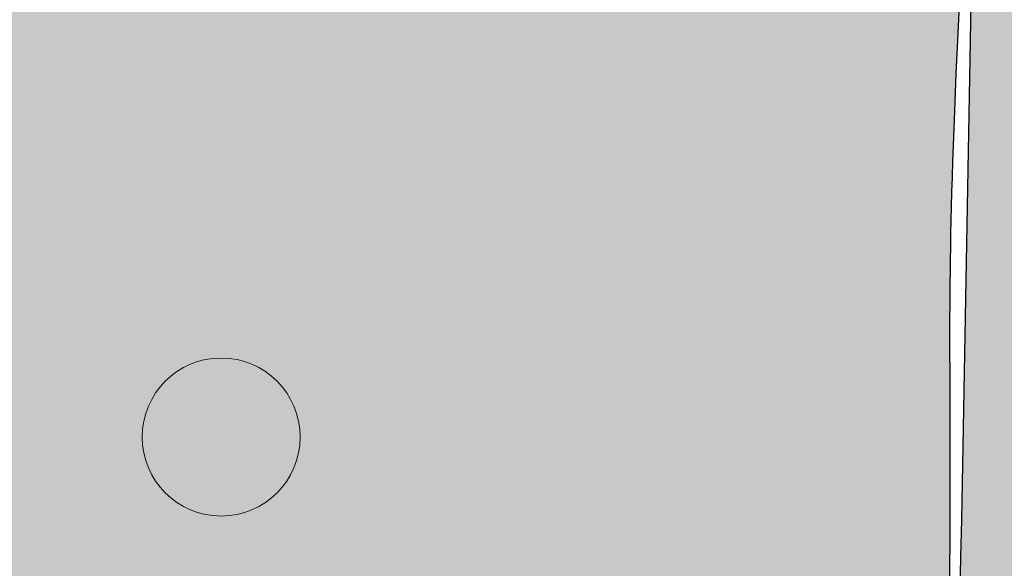
# Model space of a CAD drawing. Units: millimetres. Extents: x 11032 to 26788, y 3406 to 24505.
# Tile 58 of 78: x 16358 to 17293, y 15498 to 16019. Entities that reach past the tile are written whole.
import ezdxf

# ---------------------------------------------------------------- set-up
doc = ezdxf.new("R2010")
doc.units = ezdxf.units.MM
doc.header["$MEASUREMENT"] = 0
for name, color, linetype, lineweight in [('A-ANNO-DIMS', 2, 'Continuous', 18), ('A-ELEV-GUIT', 7, 'Continuous', 18), ('A-ROOF', 7, 'Continuous', 30), ('A-WALL', 7, 'Continuous', 35), ('E-LITE', 7, 'Continuous', 18), ('E-LITE-PATT', 7, 'Continuous', 13)]:
    doc.layers.add(name, color=color, linetype=linetype, lineweight=lineweight)
doc.layers.add('A-ROOF-PATT', color=9, linetype='Continuous', lineweight=13, true_color=0xc7c8ca)
doc.styles.get("Standard").update_dxf_attribs({"font": 'arial.ttf'})
doc.dimstyles.get("Standard").update_dxf_attribs({"dimtxt": 150, "dimasz": 100, "dimexe": 10, "dimexo": 5, "dimgap": 5, "dimtad": 0, "dimtih": 1, "dimtoh": 1, "dimdec": 0, "dimzin": 0, "dimdsep": 46, "dimtxsty": 'Standard', "dimcen": 0.09, "dimadec": 0, "dimazin": 0, "dimtfac": 1, "dimtdec": 0, "dimtofl": 0, "dimtmove": 0, "dimatfit": 3, "dimfxl": 1, "dimtolj": 1, "dimtzin": 0, "dimarcsym": 0})

# ---------------------------------------------------------------- blocks, each defined once
blk = doc.blocks.new('RECESSED-LIGHT-150')
blk.add_circle((75, 75), 75)
blk = doc.blocks.new('*D36')
at = {"layer": 'A-ANNO-DIMS', "color": 0, "lineweight": -2, "transparency": 16777216}
for p, q in [((12301.26, 17115.89), (12301.26, 24416.86)), ((25397.4, 4466.4), (25397.4, 24416.86)), ((12401.26, 24406.86), (18569.2, 24406.86)), ((25297.4, 24406.86), (19129.47, 24406.86))]:
    blk.add_line(p, q, dxfattribs=at)
at = {"layer": 'A-ANNO-DIMS', "color": 0, "transparency": 16777216}
for points in [[(12401.26, 24423.52), (12401.26, 24390.19), (12301.26, 24406.86)], [(25297.4, 24423.52), (25297.4, 24390.19), (25397.4, 24406.86)]]:
    blk.add_solid(points, dxfattribs=at)
at = {"layer": 'Defpoints', "color": 0, "transparency": 16777216}
for p in [(25397.4, 24406.86), (12301.26, 17110.89), (25397.4, 4461.4)]:
    blk.add_point(p, dxfattribs=at)
at = {"layer": 'A-ANNO-DIMS', "color": 0, "transparency": 16777216, "insert": (18849.33, 24406.86), "char_height": 150, "attachment_point": 5}
blk.add_mtext('\\A1;13096', dxfattribs=at)
blk = doc.blocks.new('*D37')
at = {"layer": 'A-ANNO-DIMS', "color": 0, "lineweight": -2, "transparency": 16777216}
for p, q in [((18087.74, 23450.36), (11334.76, 23450.36)), ((11344.76, 23350.36), (11344.76, 14037.46)), ((11344.76, 4561.4), (11344.76, 13874.29)), ((12927.66, 4461.4), (11334.76, 4461.4))]:
    blk.add_line(p, q, dxfattribs=at)
at = {"layer": 'A-ANNO-DIMS', "color": 0, "transparency": 16777216}
for points in [[(11328.1, 23350.36), (11361.43, 23350.36), (11344.76, 23450.36)], [(11328.1, 4561.4), (11361.43, 4561.4), (11344.76, 4461.4)]]:
    blk.add_solid(points, dxfattribs=at)
at = {"layer": 'Defpoints', "color": 0, "transparency": 16777216}
for p in [(11344.76, 23450.36), (18092.74, 23450.36), (12932.66, 4461.4)]:
    blk.add_point(p, dxfattribs=at)
at = {"layer": 'A-ANNO-DIMS', "color": 0, "transparency": 16777216, "insert": (11344.76, 13955.88), "char_height": 150, "attachment_point": 5}
blk.add_mtext('\\A1;18989', dxfattribs=at)
blk = doc.blocks.new('*D57')
at = {"layer": 'A-ANNO-DIMS', "color": 0, "lineweight": -2, "transparency": 16777216}
for p, q in [((14994.7, 7266.4), (14994.7, 24416.86)), ((20894.7, 7266.4), (20894.7, 24416.86)), ((15094.7, 24406.86), (17715.98, 24406.86)), ((20794.7, 24406.86), (18173.42, 24406.86))]:
    blk.add_line(p, q, dxfattribs=at)
at = {"layer": 'A-ANNO-DIMS', "color": 0, "transparency": 16777216}
for points in [[(15094.7, 24423.52), (15094.7, 24390.19), (14994.7, 24406.86)], [(20794.7, 24423.52), (20794.7, 24390.19), (20894.7, 24406.86)]]:
    blk.add_solid(points, dxfattribs=at)
at = {"layer": 'Defpoints', "color": 0, "transparency": 16777216}
for p in [(20894.7, 24406.86), (14994.7, 7261.4), (20894.7, 7261.4)]:
    blk.add_point(p, dxfattribs=at)
at = {"layer": 'A-ANNO-DIMS', "color": 0, "transparency": 16777216, "insert": (17944.7, 24406.86), "char_height": 150, "attachment_point": 5}
blk.add_mtext('\\A1;5900', dxfattribs=at)

msp = doc.modelspace()

# ---------------------------------------------------------------- hatches: boundary and pattern name
at = {"layer": 'A-ROOF-PATT'}
h = msp.add_hatch(color=256, dxfattribs=at)
edge = h.paths.add_edge_path()
edge.add_spline(control_points=[(17532.827, 17324.837), (17391.335, 17349.016), (16840.872, 17494.912), (16080.055, 18069.544), (14738.803, 18299.641), (13382.429, 18838.336), (12580.532, 17870.207), (12430.422, 17563.822)], knot_values=[2977.6027945, 2977.6027945, 2977.6027945, 2977.6027945, 3438.1840601, 4811.6463022, 5622.8675483, 7588.0288188, 8560.6685791, 8560.6685791, 8560.6685791, 8560.6685791], degree=3, periodic=0)
edge.add_spline(control_points=[(12430.422, 17563.822), (12437.904, 17573.36), (12445.386, 17582.899), (12452.869, 17592.437), (12452.869, 17592.438), (12452.869, 17592.438), (12452.869, 17592.438)], knot_values=[1408.564138, 1408.564138, 1408.564138, 1408.564138, 1444.85989, 1444.85989, 1444.85989, 1444.8601183, 1444.8601183, 1444.8601183, 1444.8601183], degree=3, periodic=0)
edge.add_spline(control_points=[(12452.869, 17592.438), (12555.432, 17723.185), (12736.557, 17929.686), (13044.86, 18114.643), (13219.943, 18189.644), (13299.92, 18220.646)], knot_values=[339.318246, 339.318246, 339.318246, 339.318246, 836.8349967, 1151.2512933, 1408.564138, 1408.564138, 1408.564138, 1408.564138], degree=3, periodic=0)
edge.add_spline(control_points=[(13299.92, 18220.646), (13299.998, 18220.689), (13300.077, 18220.732), (13319.738, 18231.488), (13339.24, 18241.402), (13388.645, 18264.703), (13418.466, 18277.069), (13478.019, 18298.648), (13507.751, 18307.861), (13544.561, 18317.488), (13551.584, 18319.245), (13558.612, 18320.924)], knot_values=[3783.8950972, 3783.8950972, 3783.8950972, 3783.8950972, 3784.1737101, 3784.1737101, 3853.4666747, 3853.4666747, 3960.2401917, 3960.2401917, 4067.0137087, 4067.0137087, 4092.1744649, 4092.1744649, 4092.1744649, 4092.1744649], degree=3, periodic=0)
edge.add_spline(control_points=[(13558.612, 18320.924), (13581.407, 18326.373), (13604.25, 18331.007), (13657.184, 18339.957), (13687.338, 18343.732), (13748.098, 18348.892), (13778.704, 18350.276), (13840.46, 18350.833), (13871.609, 18350.005), (13934.496, 18346.313), (13966.232, 18343.449), (14030.297, 18335.871), (14062.625, 18331.158), (14127.853, 18320.088), (14160.753, 18313.73), (14241.357, 18296.556), (14289.343, 18284.997), (14386.31, 18259.688), (14435.291, 18245.941), (14534.161, 18217.034), (14584.049, 18201.875), (14684.682, 18170.964), (14735.427, 18155.212), (14837.763, 18123.971), (14889.354, 18108.482), (14954.971, 18089.677), (14968.586, 18085.823), (14992.391, 18079.184), (15002.566, 18076.376), (15021.739, 18071.153), (15030.731, 18068.729), (15047.707, 18064.21), (15055.694, 18062.106), (15079.815, 18055.825), (15095.905, 18051.728), (15143.966, 18039.717), (15175.729, 18032.084), (15254.84, 18013.501), (15301.798, 18002.866), (15394.186, 17981.845), (15439.615, 17971.459), (15528.833, 17950.135), (15572.62, 17939.197), (15658.477, 17916.021), (15700.546, 17903.785), (15753.633, 17886.734), (15765.446, 17882.835), (15786.574, 17875.653), (15795.915, 17872.404), (15810.108, 17867.349), (15814.99, 17865.588), (15824.736, 17862.029), (15829.611, 17860.226), (15844.241, 17854.75), (15854.002, 17851.008), (15883.312, 17839.521), (15902.885, 17831.512), (15966.355, 17804.548), (16010.39, 17784.302), (16098.838, 17741.267), (16143.25, 17718.478), (16232.497, 17671.098), (16277.332, 17646.507), (16367.515, 17596.295), (16412.862, 17570.676), (16504.202, 17519.209), (16550.194, 17493.362), (16643.009, 17442.263), (16689.831, 17417.011), (16756.517, 17382.472), (16775.937, 17372.58), (16795.455, 17362.84)], knot_values=[4092.1744649, 4092.1744649, 4092.1744649, 4092.1744649, 4173.7872258, 4173.7872258, 4280.5607428, 4280.5607428, 4387.3342598, 4387.3342598, 4494.1077768, 4494.1077768, 4600.8812939, 4600.8812939, 4707.6548109, 4707.6548109, 4814.4283279, 4814.4283279, 4967.1262405, 4967.1262405, 5119.8241531, 5119.8241531, 5272.5220657, 5272.5220657, 5425.2199783, 5425.2199783, 5577.9178908, 5577.9178908, 5617.7853319, 5617.7853319, 5647.4648479, 5647.4648479, 5673.611025, 5673.611025, 5696.747607, 5696.747607, 5743.6818903, 5743.6818903, 5837.5504571, 5837.5504571, 5979.7261046, 5979.7261046, 6121.9017521, 6121.9017521, 6264.0773996, 6264.0773996, 6406.2530471, 6406.2530471, 6447.2585849, 6447.2585849, 6480.0420882, 6480.0420882, 6497.3077062, 6497.3077062, 6514.5733242, 6514.5733242, 6549.1045602, 6549.1045602, 6618.1670322, 6618.1670322, 6772.6610171, 6772.6610171, 6927.155002, 6927.155002, 7081.6489869, 7081.6489869, 7236.1429718, 7236.1429718, 7390.6369567, 7390.6369567, 7545.1309416, 7545.1309416, 7608.1992868, 7608.1992868, 7608.1992868, 7608.1992868], degree=3, periodic=0)
edge.add_spline(control_points=[(16795.455, 17362.84), (16814.335, 17349.456), (16832.897, 17336.263), (16873.225, 17307.197), (16894.778, 17291.386), (16936.221, 17259.941), (16956.11, 17244.308), (16993.863, 17213.094), (17011.726, 17197.514), (17041.993, 17169.265), (17054.791, 17156.601), (17078.762, 17131.225), (17089.933, 17118.516), (17110.618, 17092.991), (17120.131, 17080.178), (17130.17, 17065.264), (17131.487, 17063.277), (17133.77, 17059.776), (17134.746, 17058.261), (17136.69, 17055.205), (17137.657, 17053.668), (17140.539, 17049.025), (17142.438, 17045.89), (17148.068, 17036.367), (17151.732, 17029.859), (17163.03, 17008.788), (17170.335, 16993.646), (17184.087, 16961.978), (17190.534, 16945.453), (17202.562, 16911.165), (17208.142, 16893.402), (17218.448, 16856.821), (17223.173, 16838.003), (17231.801, 16799.51), (17235.705, 16779.837), (17241.533, 16746.739), (17243.676, 16733.5), (17247.718, 16706.37), (17249.608, 16692.472), (17252.066, 16672.69), (17252.761, 16666.875), (17254.1, 16655.226), (17254.744, 16649.4), (17256.596, 16631.917), (17257.727, 16620.254), (17260.823, 16585.238), (17262.489, 16561.858), (17266.551, 16488.654), (17267.658, 16438.661), (17267.349, 16375.228), (17267.193, 16362.07), (17266.95, 16348.891)], knot_values=[15.1130472, 15.1130472, 15.1130472, 15.1130472, 82.6995146, 82.6995146, 165.3990291, 165.3990291, 248.0985437, 248.0985437, 330.7980583, 330.7980583, 397.9419458, 397.9419458, 465.0858333, 465.0858333, 532.2297209, 532.2297209, 542.533741, 542.533741, 550.3568158, 550.3568158, 558.1798906, 558.1798906, 573.8260402, 573.8260402, 605.1183395, 605.1183395, 672.7640614, 672.7640614, 740.4097834, 740.4097834, 808.0555054, 808.0555054, 875.7012273, 875.7012273, 943.3469493, 943.3469493, 987.6613492, 987.6613492, 1033.4121612, 1033.4121612, 1052.3850876, 1052.3850876, 1071.358014, 1071.358014, 1109.3038668, 1109.3038668, 1185.1955724, 1185.1955724, 1346.4419026, 1346.4419026, 1388.5586631, 1388.5586631, 1388.5586631, 1388.5586631], degree=3, periodic=0)
edge.add_spline(control_points=[(17266.95, 16348.891), (17266.95, 16348.891), (17266.95, 16348.891), (17266.95, 16348.891), (17253.182, 15602.417), (17239.414, 14855.943), (17225.646, 14109.469)], knot_values=[1388.5586631, 1388.5586631, 1388.5586631, 1388.5586631, 1388.5589654, 1388.5589654, 1388.5589654, 3774.0767661, 3774.0767661, 3774.0767661, 3774.0767661], degree=3, periodic=0)
edge.add_spline(control_points=[(17225.646, 14109.469), (17226.198, 14109.827), (17226.748, 14110.185), (17242.065, 14120.191), (17255.956, 14130.116), (17274.422, 14144.286), (17279.609, 14148.386), (17284.686, 14152.511)], knot_values=[1926.3423968, 1926.3423968, 1926.3423968, 1926.3423968, 1927.316729, 1927.316729, 1953.5121761, 1953.5121761, 1964.0732348, 1964.0732348, 1964.0732348, 1964.0732348], degree=3, periodic=0)
edge.add_spline(control_points=[(17284.686, 14152.511), (17315.791, 14194.761), (17384.413, 14446.273), (17407.128, 14793.401), (17407.093, 15295.84), (17423.274, 15626.362), (17415.601, 15782.507)], knot_values=[0, 0, 0, 0, 163.2554674, 619.2296767, 1171.8624483, 1621.6355562, 1621.6355562, 1621.6355562, 1621.6355562], degree=3, periodic=0)
edge.add_spline(control_points=[(17415.601, 15782.507), (17438.21, 16077.57), (17410.495, 16533.484), (17390.893, 17030.649), (17301.082, 17169.349)], knot_values=[543.9784753, 543.9784753, 543.9784753, 543.9784753, 1452.9852767, 1960.0114926, 1960.0114926, 1960.0114926, 1960.0114926], degree=3, periodic=0)
edge.add_spline(control_points=[(17301.082, 17169.349), (17346.58, 17157.64), (17392.235, 17147.336), (17467.161, 17132.609), (17496.336, 17127.412), (17525.58, 17122.709)], knot_values=[8131.593939, 8131.593939, 8131.593939, 8131.593939, 8269.7349273, 8269.7349273, 8357.5016646, 8357.5016646, 8357.5016646, 8357.5016646], degree=3, periodic=0)
edge.add_line((17525.58, 17122.709), (17532.827, 17324.837))
edge = h.paths.add_edge_path(flags=17)
edge.add_spline(control_points=[(13340.537, 14602.706), (13316.172, 14726.456), (13323.666, 14932.342), (13637.836, 15081.117), (13863.248, 15171.051), (14002.1, 15224.503), (14058.539, 15244.876)], knot_values=[680.8931862, 680.8931862, 680.8931862, 680.8931862, 1033.4728289, 1337.4008326, 1604.7214264, 1784.2944722, 1784.2944722, 1784.2944722, 1784.2944722], degree=3, periodic=0)
edge.add_spline(control_points=[(14058.539, 15244.876), (14058.289, 15275.236), (14057.634, 15305.434), (14055.312, 15376.527), (14053.359, 15417.248), (14048.642, 15497.048), (14045.89, 15536.143), (14042.888, 15574.619)], knot_values=[6573.1065419, 6573.1065419, 6573.1065419, 6573.1065419, 6636.7330012, 6636.7330012, 6723.8890547, 6723.8890547, 6809.6328771, 6809.6328771, 6809.6328771, 6809.6328771], degree=3, periodic=0)
edge.add_spline(control_points=[(14042.888, 15574.619), (13546.54, 15403.221), (13074.735, 15143.241), (13277.36, 14695.339), (13340.537, 14602.706)], knot_values=[503.7925783, 503.7925783, 503.7925783, 503.7925783, 1728.1787606, 2051.34844, 2051.34844, 2051.34844, 2051.34844], degree=3, periodic=0)
h = msp.add_hatch(color=256, dxfattribs=at)
h.set_gradient(color1=(254, 234, 185), color2=(254, 204, 102), name='HEMISPHERICAL')
edge = h.paths.add_edge_path()
edge.add_line((15084.393, 17001.32), (15284.393, 17051.32))
edge.add_line((15284.393, 17051.32), (15470.537, 16752.334))
edge.add_spline(control_points=[(15470.537, 16752.334), (15683.311, 16831.508), (16106.827, 16912.335), (16625.609, 16876.997), (17083.498, 16357.78), (17257.801, 16180.113)], knot_values=[0, 0, 0, 0, 655.2936334, 1252.0157838, 1989.6162859, 1989.6162859, 1989.6162859, 1989.6162859], degree=3, periodic=0)
edge.add_spline(control_points=[(17257.801, 16180.113), (17260.851, 16236.372), (17263.9, 16292.632), (17266.95, 16348.891)], knot_values=[1132.9967717, 1132.9967717, 1132.9967717, 1132.9967717, 1198.0464225, 1198.0464225, 1198.0464225, 1198.0464225], degree=3, periodic=0)
edge.add_spline(control_points=[(17266.95, 16348.891), (17267.193, 16362.07), (17267.349, 16375.228), (17267.658, 16438.661), (17266.551, 16488.654), (17262.489, 16561.858), (17260.823, 16585.238), (17257.727, 16620.254), (17256.596, 16631.917), (17254.744, 16649.4), (17254.1, 16655.226), (17252.761, 16666.875), (17252.066, 16672.69), (17249.608, 16692.472), (17247.718, 16706.37), (17243.676, 16733.5), (17241.533, 16746.739), (17235.705, 16779.837), (17231.801, 16799.51), (17223.173, 16838.003), (17218.448, 16856.821), (17208.142, 16893.402), (17202.562, 16911.165), (17190.534, 16945.453), (17184.087, 16961.978), (17170.335, 16993.646), (17163.03, 17008.788), (17151.732, 17029.859), (17148.068, 17036.367), (17142.438, 17045.89), (17140.539, 17049.025), (17137.657, 17053.668), (17136.69, 17055.205), (17134.746, 17058.261), (17133.77, 17059.776), (17131.487, 17063.277), (17130.17, 17065.264), (17120.131, 17080.178), (17110.618, 17092.991), (17089.933, 17118.516), (17078.762, 17131.225), (17054.791, 17156.601), (17041.993, 17169.265), (17011.726, 17197.514), (16993.863, 17213.094), (16956.11, 17244.308), (16936.221, 17259.941), (16894.778, 17291.386), (16873.225, 17307.197), (16832.897, 17336.263), (16814.335, 17349.456), (16795.455, 17362.84)], knot_values=[15.1130472, 15.1130472, 15.1130472, 15.1130472, 57.2298077, 57.2298077, 218.4761379, 218.4761379, 294.3678435, 294.3678435, 332.3136963, 332.3136963, 351.2866227, 351.2866227, 370.2595491, 370.2595491, 416.0103612, 416.0103612, 460.324761, 460.324761, 527.970483, 527.970483, 595.616205, 595.616205, 663.2619269, 663.2619269, 730.9076489, 730.9076489, 798.5533709, 798.5533709, 829.8456701, 829.8456701, 845.4918197, 845.4918197, 853.3148945, 853.3148945, 861.1379693, 861.1379693, 871.4419895, 871.4419895, 938.585877, 938.585877, 1005.7297645, 1005.7297645, 1072.8736521, 1072.8736521, 1155.5731666, 1155.5731666, 1238.2726812, 1238.2726812, 1320.9721958, 1320.9721958, 1388.5586631, 1388.5586631, 1388.5586631, 1388.5586631], degree=3, periodic=0)
edge.add_spline(control_points=[(16795.455, 17362.84), (16775.937, 17372.58), (16756.517, 17382.472), (16689.831, 17417.011), (16643.009, 17442.263), (16550.194, 17493.362), (16504.202, 17519.209), (16412.862, 17570.676), (16367.515, 17596.295), (16277.332, 17646.507), (16232.497, 17671.098), (16143.25, 17718.478), (16098.838, 17741.267), (16010.39, 17784.302), (15966.355, 17804.548), (15902.885, 17831.512), (15883.312, 17839.521), (15854.002, 17851.008), (15844.241, 17854.75), (15829.611, 17860.226), (15824.736, 17862.029), (15814.99, 17865.588), (15810.108, 17867.349), (15795.915, 17872.404), (15786.574, 17875.653), (15765.446, 17882.835), (15753.633, 17886.734), (15700.546, 17903.785), (15658.477, 17916.021), (15572.62, 17939.197), (15528.833, 17950.135), (15439.615, 17971.459), (15394.186, 17981.845), (15301.798, 18002.866), (15254.84, 18013.501), (15175.729, 18032.084), (15143.966, 18039.717), (15095.905, 18051.728), (15079.815, 18055.825), (15055.694, 18062.106), (15047.707, 18064.21), (15030.731, 18068.729), (15021.739, 18071.153), (15002.566, 18076.376), (14992.391, 18079.184), (14968.586, 18085.823), (14954.971, 18089.677), (14889.354, 18108.482), (14837.763, 18123.971), (14735.427, 18155.212), (14684.682, 18170.964), (14584.049, 18201.875), (14534.161, 18217.034), (14435.291, 18245.941), (14386.31, 18259.688), (14289.343, 18284.997), (14241.357, 18296.556), (14160.753, 18313.73), (14127.853, 18320.088), (14062.625, 18331.158), (14030.297, 18335.871), (13966.232, 18343.449), (13934.496, 18346.313), (13871.609, 18350.005), (13840.46, 18350.833), (13778.704, 18350.276), (13748.098, 18348.892), (13687.338, 18343.732), (13657.184, 18339.957), (13604.25, 18331.007), (13581.407, 18326.373), (13558.612, 18320.924)], knot_values=[4092.1744649, 4092.1744649, 4092.1744649, 4092.1744649, 4155.2428101, 4155.2428101, 4309.736795, 4309.736795, 4464.2307799, 4464.2307799, 4618.7247648, 4618.7247648, 4773.2187497, 4773.2187497, 4927.7127346, 4927.7127346, 5082.2067195, 5082.2067195, 5151.2691915, 5151.2691915, 5185.8004275, 5185.8004275, 5203.0660455, 5203.0660455, 5220.3316635, 5220.3316635, 5253.1151668, 5253.1151668, 5294.1207046, 5294.1207046, 5436.2963521, 5436.2963521, 5578.4719996, 5578.4719996, 5720.6476471, 5720.6476471, 5862.8232946, 5862.8232946, 5956.6918614, 5956.6918614, 6003.6261447, 6003.6261447, 6026.7627267, 6026.7627267, 6052.9089038, 6052.9089038, 6082.5884198, 6082.5884198, 6122.4558609, 6122.4558609, 6275.1537734, 6275.1537734, 6427.851686, 6427.851686, 6580.5495986, 6580.5495986, 6733.2475112, 6733.2475112, 6885.9454238, 6885.9454238, 6992.7189408, 6992.7189408, 7099.4924578, 7099.4924578, 7206.2659749, 7206.2659749, 7313.0394919, 7313.0394919, 7419.8130089, 7419.8130089, 7526.5865259, 7526.5865259, 7608.1992868, 7608.1992868, 7608.1992868, 7608.1992868], degree=3, periodic=0)
edge.add_spline(control_points=[(13558.612, 18320.924), (13472.381, 18287.498), (13386.15, 18254.072), (13299.92, 18220.646), (13299.92, 18220.646), (13299.92, 18220.646), (13299.92, 18220.646)], knot_values=[61.8832457, 61.8832457, 61.8832457, 61.8832457, 339.3179746, 339.3179746, 339.3179746, 339.318246, 339.318246, 339.318246, 339.318246], degree=3, periodic=0)
edge.add_spline(control_points=[(13299.92, 18220.646), (13219.943, 18189.644), (13044.86, 18114.643), (12736.557, 17929.686), (12555.432, 17723.185), (12452.869, 17592.438)], knot_values=[339.318246, 339.318246, 339.318246, 339.318246, 596.6310906, 911.0473872, 1408.564138, 1408.564138, 1408.564138, 1408.564138], degree=3, periodic=0)
edge.add_spline(control_points=[(12452.869, 17592.438), (12452.869, 17592.438), (12452.869, 17592.438), (12452.869, 17592.437), (12445.386, 17582.899), (12437.904, 17573.36), (12430.422, 17563.822)], knot_values=[1408.564138, 1408.564138, 1408.564138, 1408.564138, 1408.5643663, 1408.5643663, 1408.5643663, 1444.8601183, 1444.8601183, 1444.8601183, 1444.8601183], degree=3, periodic=0)
edge.add_spline(control_points=[(12430.422, 17563.822), (12373.797, 17448.248), (12157.302, 16836.764), (12751.985, 16393.69), (13424.325, 15907.903), (14042.888, 15574.619)], knot_values=[0, 0, 0, 0, 366.8993034, 1975.5941082, 2977.6027945, 2977.6027945, 2977.6027945, 2977.6027945], degree=3, periodic=0)
edge.add_spline(control_points=[(14042.888, 15574.619), (14042.839, 15575.252), (14042.789, 15575.886), (14039.681, 15615.607), (14036.366, 15654.052), (14029.551, 15729.305), (14026.05, 15766.114), (14019.175, 15837.686), (14015.8, 15872.45), (13903.823, 16338.596)], knot_values=[6310.2261504, 6310.2261504, 6310.2261504, 6310.2261504, 6311.6383814, 6311.6383814, 6398.7944349, 6398.7944349, 6485.9504884, 6485.9504884, 6573.1065419, 6573.1065419, 6573.1065419, 6573.1065419], degree=3, periodic=0)
edge.add_spline(control_points=[(13903.823, 16338.596), (14237.315, 16236.889), (14456.623, 16167.555), (14614.196, 16115.84)], knot_values=[0, 0, 0, 0, 202.9853419, 202.9853419, 202.9853419, 202.9853419], degree=3, periodic=0)
edge.add_spline(control_points=[(14614.196, 16115.84), (14663.209, 16178.992), (14799.965, 16341.237), (14969.915, 16481.426), (15084.393, 16556.825)], knot_values=[2405.0345045, 2405.0345045, 2405.0345045, 2405.0345045, 2644.8826966, 3039.2707272, 3039.2707272, 3039.2707272, 3039.2707272], degree=3, periodic=0)
edge.add_line((15084.393, 16556.825), (15084.393, 17001.32))
h.paths.add_polyline_path([(14195.599, 17606.181, -1), (14395.599, 17606.181, -1)], flags=16)
h.paths.add_polyline_path([(13310.178, 17032.97, -1), (13510.178, 17032.97, -1)], flags=16)
h = msp.add_hatch(color=256, dxfattribs=at)
h.set_gradient(color1=(254, 234, 185), color2=(254, 204, 102), name='HEMISPHERICAL')
edge = h.paths.add_edge_path()
edge.add_spline(control_points=[(16560.042, 14907.752), (16569.192, 14907.664), (16578.343, 14907.575), (16587.493, 14907.486), (16832.101, 14905.115), (17122.895, 14902.296), (16849.359, 14976.117), (16870.954, 15304.114), (17098.337, 15241.178), (17235.385, 15203.245)], knot_values=[0, 0, 0, 0, 14.8674385, 14.8674385, 14.8674385, 412.2943091, 487.3345915, 708.6416004, 1044.3939449, 1044.3939449, 1044.3939449, 1044.3939449], degree=3, periodic=0)
edge.add_line((16587.504, 14907.486), (16560.207, 14907.486))
edge.add_line((16560.207, 14907.486), (15784.393, 16153.61))
edge.add_line((15784.393, 16153.61), (15784.393, 15385.996))
edge.add_spline(control_points=[(15784.393, 15385.996), (15798.391, 15360.52), (15847.198, 15266.214), (15887.196, 15168.614), (15912.903, 15096.727)], knot_values=[1463.2850479, 1463.2850479, 1463.2850479, 1463.2850479, 1550.659771, 1779.9599361, 1779.9599361, 1779.9599361, 1779.9599361], degree=3, periodic=0)
edge.add_spline(control_points=[(15912.903, 15096.727), (15913.652, 15095.649), (15914.403, 15094.565), (15925.191, 15078.948), (15935.516, 15063.47), (15956.582, 15030.918), (15967.324, 15013.844), (15989.119, 14978.386), (16000.173, 14960.003), (16022.525, 14922.193), (16033.824, 14902.767), (16056.63, 14863.116), (16068.138, 14842.891), (16091.349, 14801.871), (16103.053, 14781.075), (16126.666, 14739.118), (16138.575, 14717.958), (16162.628, 14675.459), (16174.772, 14654.12), (16199.352, 14611.428), (16211.787, 14590.075), (16237.037, 14547.491), (16249.851, 14526.26), (16271.946, 14490.566), (16281.092, 14476.044), (16299.694, 14447.129), (16309.149, 14432.737), (16328.456, 14404.098), (16338.307, 14389.85), (16358.518, 14361.503), (16368.879, 14347.403), (16390.266, 14319.347), (16401.291, 14305.391), (16420.626, 14281.969), (16428.703, 14272.467), (16445.363, 14253.527), (16453.946, 14244.088), (16471.727, 14225.278), (16480.926, 14215.907), (16500.075, 14197.247), (16510.026, 14187.959), (16530.844, 14169.504), (16541.71, 14160.337), (16564.549, 14142.195), (16576.522, 14133.22), (16597.69, 14118.448), (16606.528, 14112.565), (16624.87, 14101.004), (16634.376, 14095.326), (16654.117, 14084.255), (16664.352, 14078.862), (16685.603, 14068.46), (16696.619, 14063.452), (16719.46, 14053.944), (16731.285, 14049.444), (16755.742, 14041.097), (16768.374, 14037.251), (16794.396, 14030.368), (16807.787, 14027.332), (16835.229, 14022.23), (16849.279, 14020.163), (16877.882, 14017.141), (16892.435, 14016.186), (16921.835, 14015.489), (16936.683, 14015.749), (16961.564, 14017.241), (16971.582, 14018.127), (16986.57, 14019.883), (16991.56, 14020.54), (16999.027, 14021.63), (17001.514, 14022.011), (17006.48, 14022.809), (17008.962, 14023.225), (17014.824, 14024.251), (17018.193, 14024.875), (17036.262, 14028.398), (17050.55, 14031.826), (17078.171, 14039.583), (17091.505, 14043.912), (17115.643, 14052.705), (17126.557, 14057.089), (17137.108, 14061.688)], knot_values=[2010.7639617, 2010.7639617, 2010.7639617, 2010.7639617, 2014.7029827, 2014.7029827, 2067.238337, 2067.238337, 2119.7736913, 2119.7736913, 2172.3090457, 2172.3090457, 2224.8444, 2224.8444, 2277.3797543, 2277.3797543, 2329.9151086, 2329.9151086, 2382.450463, 2382.450463, 2434.9858173, 2434.9858173, 2487.5211716, 2487.5211716, 2540.0565259, 2540.0565259, 2576.3179289, 2576.3179289, 2612.5793318, 2612.5793318, 2648.8407347, 2648.8407347, 2685.1021376, 2685.1021376, 2721.3635405, 2721.3635405, 2746.252015, 2746.252015, 2771.1404895, 2771.1404895, 2796.028964, 2796.028964, 2820.9174385, 2820.9174385, 2845.8059131, 2845.8059131, 2870.6943876, 2870.6943876, 2887.5132757, 2887.5132757, 2904.3321639, 2904.3321639, 2921.1510521, 2921.1510521, 2937.9699402, 2937.9699402, 2954.7888284, 2954.7888284, 2971.6077166, 2971.6077166, 2988.4266047, 2988.4266047, 3005.2454929, 3005.2454929, 3022.0643811, 3022.0643811, 3038.8832692, 3038.8832692, 3050.1975453, 3050.1975453, 3055.8546833, 3055.8546833, 3058.6832524, 3058.6832524, 3061.5118214, 3061.5118214, 3065.3934173, 3065.3934173, 3082.4668716, 3082.4668716, 3099.5403259, 3099.5403259, 3114.5433443, 3114.5433443, 3114.5433443, 3114.5433443], degree=3, periodic=0)
edge.add_spline(control_points=[(17137.108, 14061.688), (17165.253, 14274.398), (17209.97, 14653.885), (17230.2, 15035.586), (17235.385, 15203.245)], knot_values=[1968.0804557, 1968.0804557, 1968.0804557, 1968.0804557, 2611.5282875, 3114.5379264, 3114.5379264, 3114.5379264, 3114.5379264], degree=3, periodic=0)
edge = h.paths.add_edge_path()
edge.add_spline(control_points=[(16856.103, 14956.992), (16852.841, 14961.219), (16849.83, 14965.576), (16842.539, 14977.287), (16838.658, 14984.798), (16832.033, 15000.109), (16829.289, 15007.911), (16824.126, 15026.008), (16822.047, 15036.354), (16819.308, 15057.097), (16818.649, 15067.496), (16818.576, 15088.188), (16819.162, 15098.483), (16821.467, 15118.823), (16823.186, 15128.868), (16827.696, 15148.567), (16830.486, 15158.22), (16836.065, 15173.969), (16838.565, 15180.211), (16844.079, 15192.402), (16847.092, 15198.353), (16852.029, 15207.021), (16853.744, 15209.868), (16857.321, 15215.468), (16859.188, 15218.226), (16863.017, 15223.558), (16864.978, 15226.136), (16872.565, 15235.558), (16878.593, 15241.952), (16891.428, 15253.591), (16898.232, 15258.834), (16912.397, 15268.127), (16919.756, 15272.176), (16934.816, 15279.138), (16942.515, 15282.052), (16958.1, 15286.873), (16965.985, 15288.78), (16984.013, 15292.142), (16994.186, 15293.334), (17014.631, 15294.619), (17024.904, 15294.713), (17048.453, 15293.935), (17061.76, 15292.783), (17088.519, 15289.422), (17101.972, 15287.211), (17131.961, 15281.46), (17148.526, 15277.734), (17181.692, 15269.627), (17198.292, 15265.245), (17222.182, 15258.759), (17229.535, 15256.737), (17236.862, 15254.714)], knot_values=[9.6639535, 9.6639535, 9.6639535, 9.6639535, 20.0351668, 20.0351668, 36.9411752, 36.9411752, 53.8471837, 53.8471837, 75.7795687, 75.7795687, 97.7119538, 97.7119538, 119.6443388, 119.6443388, 141.5767238, 141.5767238, 163.5091089, 163.5091089, 178.3829945, 178.3829945, 193.2568801, 193.2568801, 200.6938229, 200.6938229, 208.1307657, 208.1307657, 215.4448585, 215.4448585, 235.5795923, 235.5795923, 255.7143261, 255.7143261, 275.8490598, 275.8490598, 295.9837936, 295.9837936, 316.1185274, 316.1185274, 341.7220543, 341.7220543, 367.3255812, 367.3255812, 400.1572431, 400.1572431, 432.988905, 432.988905, 473.0440165, 473.0440165, 513.099128, 513.099128, 530.9692999, 530.9692999, 530.9692999, 530.9692999], degree=3, periodic=0)
edge.add_spline(control_points=[(17236.862, 15254.714), (17240.377, 15387.456), (17242.496, 15609.536), (17239.752, 15831.567), (17250.544, 16044.717)], knot_values=[1250.9818616, 1250.9818616, 1250.9818616, 1250.9818616, 1649.1516581, 1916.613987, 1916.613987, 1916.613987, 1916.613987], degree=3, periodic=0)
edge.add_spline(control_points=[(17250.544, 16044.717), (17229.169, 16066.505), (17207.794, 16088.292), (17186.419, 16110.08), (17186.418, 16110.08), (17186.418, 16110.081), (17186.418, 16110.081)], knot_values=[-88.5185581, -88.5185581, -88.5185581, -88.5185581, -0.0012784, -0.0012784, -0.0012784, 0, 0, 0, 0], degree=3, periodic=0)
edge.add_spline(control_points=[(17186.418, 16110.081), (17169.261, 16127.569), (17151.499, 16145.947), (17114.892, 16184.084), (17096.046, 16203.842), (17057.437, 16244.305), (17037.673, 16265.01), (16997.415, 16306.918), (16976.921, 16328.12), (16927.79, 16378.347), (16898.924, 16407.388), (16840.771, 16464.327), (16811.484, 16492.225), (16758.449, 16540.764), (16734.666, 16561.798), (16687.634, 16601.588), (16664.382, 16620.344), (16624.116, 16650.909), (16606.897, 16663.324), (16583.769, 16678.999), (16577.49, 16683.149), (16567.144, 16689.805), (16563.039, 16692.397), (16550.823, 16699.959), (16542.775, 16704.739), (16526.841, 16713.814), (16518.956, 16718.108), (16495.524, 16730.301), (16480.199, 16737.514), (16449.97, 16750.334), (16435.066, 16755.942), (16405.476, 16765.764), (16390.79, 16769.979), (16361.418, 16777.195), (16346.731, 16780.197), (16317.147, 16785.133), (16302.249, 16787.067), (16272.053, 16789.992), (16256.756, 16790.981), (16225.609, 16792.125), (16209.759, 16792.279), (16177.385, 16791.865), (16160.862, 16791.296), (16136.98, 16790.07), (16129.942, 16789.661), (16118.22, 16788.91), (16113.574, 16788.594), (16103.645, 16787.886), (16098.362, 16787.489), (16087.761, 16786.652), (16082.439, 16786.212), (16066.413, 16784.825), (16055.649, 16783.812), (16023.135, 16780.505), (16001.164, 16777.942), (15934.539, 16769.141), (15889.17, 16761.791), (15797.417, 16743.949), (15751.033, 16733.457), (15645.217, 16705.796), (15585.74, 16687.58), (15526.207, 16666.217), (15525.367, 16665.915), (15524.528, 16665.613)], knot_values=[0, 0, 0, 0, 71.0501454, 71.0501454, 142.1002909, 142.1002909, 213.1504363, 213.1504363, 284.2005818, 284.2005818, 381.323193, 381.323193, 478.4458043, 478.4458043, 557.8219847, 557.8219847, 637.1981651, 637.1981651, 698.3122593, 698.3122593, 721.3971375, 721.3971375, 736.7790891, 736.7790891, 767.5429924, 767.5429924, 798.3068957, 798.3068957, 859.8347022, 859.8347022, 921.3625088, 921.3625088, 982.8903154, 982.8903154, 1044.4181219, 1044.4181219, 1105.9459285, 1105.9459285, 1167.4737351, 1167.4737351, 1229.0015416, 1229.0015416, 1290.5293482, 1290.5293482, 1315.8990035, 1315.8990035, 1332.3812792, 1332.3812792, 1350.9052657, 1350.9052657, 1369.4292522, 1369.4292522, 1406.4772252, 1406.4772252, 1480.5731712, 1480.5731712, 1628.7650633, 1628.7650633, 1776.9569554, 1776.9569554, 1966.3109251, 1966.3109251, 1969.019495, 1969.019495, 1969.019495, 1969.019495], degree=3, periodic=0)
edge.add_line((15524.528, 16665.613), (16587.978, 14957.484))
edge.add_spline(control_points=[(16587.978, 14957.484), (16605.253, 14957.316), (16622.516, 14957.149), (16665.945, 14956.759), (16691.933, 14956.554), (16742.419, 14956.302), (16766.918, 14956.255), (16813.531, 14956.412), (16835.647, 14956.617), (16856.103, 14956.992)], knot_values=[872.2181925, 872.2181925, 872.2181925, 872.2181925, 900.2857301, 900.2857301, 943.3659889, 943.3659889, 986.4462476, 986.4462476, 1029.5265064, 1029.5265064, 1029.5265064, 1029.5265064], degree=3, periodic=0)
h.paths.add_polyline_path([(16474.605, 15622.642, -1), (16624.605, 15622.642, -1)], flags=16)
h.paths.add_polyline_path([(16198.536, 16037.613, -1), (16348.536, 16037.613, -1)], flags=16)
h.paths.add_polyline_path([(16475.717, 16408.125, -1), (16625.717, 16408.125, -1)], flags=16)
at = {"layer": 'E-LITE-PATT'}
h = msp.add_hatch(color=256, dxfattribs=at)
h.paths.add_polyline_path([(13510.178, 17032.97, 1), (13310.178, 17032.97, 1)])
h.paths.add_polyline_path([(14395.599, 17606.181, 1), (14195.599, 17606.181, 1)])
h.paths.add_polyline_path([(16625.717, 16408.125, 1), (16475.717, 16408.125, 1)])
h.paths.add_polyline_path([(16348.536, 16037.613, 1), (16198.536, 16037.613, 1)])
h.paths.add_polyline_path([(16624.605, 15622.642, 1), (16474.605, 15622.642, 1)])
edge = h.paths.add_edge_path()
edge.add_spline(control_points=[(17236.862, 15254.714), (17229.535, 15256.737), (17222.182, 15258.759), (17198.292, 15265.245), (17181.692, 15269.627), (17148.526, 15277.734), (17131.961, 15281.46), (17101.972, 15287.211), (17088.519, 15289.422), (17061.76, 15292.783), (17048.453, 15293.935), (17024.904, 15294.713), (17014.631, 15294.619), (16994.186, 15293.334), (16984.013, 15292.142), (16965.985, 15288.78), (16958.1, 15286.873), (16942.515, 15282.052), (16934.816, 15279.138), (16919.756, 15272.176), (16912.397, 15268.127), (16898.232, 15258.834), (16891.428, 15253.591), (16878.593, 15241.952), (16872.565, 15235.558), (16864.978, 15226.136), (16863.017, 15223.558), (16859.188, 15218.226), (16857.321, 15215.468), (16853.744, 15209.868), (16852.029, 15207.021), (16847.092, 15198.353), (16844.079, 15192.402), (16838.565, 15180.211), (16836.065, 15173.969), (16830.486, 15158.22), (16827.696, 15148.567), (16823.186, 15128.868), (16821.467, 15118.823), (16819.162, 15098.483), (16818.576, 15088.188), (16818.649, 15067.496), (16819.308, 15057.097), (16822.047, 15036.354), (16824.126, 15026.008), (16829.289, 15007.911), (16832.033, 15000.109), (16838.658, 14984.798), (16842.539, 14977.287), (16849.83, 14965.576), (16852.841, 14961.219), (16856.103, 14956.992)], knot_values=[9.6639535, 9.6639535, 9.6639535, 9.6639535, 27.5341253, 27.5341253, 67.5892368, 67.5892368, 107.6443483, 107.6443483, 140.4760102, 140.4760102, 173.3076721, 173.3076721, 198.911199, 198.911199, 224.5147259, 224.5147259, 244.6494597, 244.6494597, 264.7841935, 264.7841935, 284.9189272, 284.9189272, 305.053661, 305.053661, 325.1883948, 325.1883948, 332.5024876, 332.5024876, 339.9394304, 339.9394304, 347.3763732, 347.3763732, 362.2502588, 362.2502588, 377.1241444, 377.1241444, 399.0565295, 399.0565295, 420.9889145, 420.9889145, 442.9212995, 442.9212995, 464.8536846, 464.8536846, 486.7860696, 486.7860696, 503.6920781, 503.6920781, 520.5980866, 520.5980866, 530.9692999, 530.9692999, 530.9692999, 530.9692999], degree=3, periodic=0)
edge.add_spline(control_points=[(16856.103, 14956.992), (16835.647, 14956.617), (16813.531, 14956.412), (16766.918, 14956.255), (16742.419, 14956.302), (16691.933, 14956.554), (16665.945, 14956.759), (16622.516, 14957.149), (16605.253, 14957.316), (16587.978, 14957.484)], knot_values=[872.2181925, 872.2181925, 872.2181925, 872.2181925, 915.2984513, 915.2984513, 958.37871, 958.37871, 1001.4589687, 1001.4589687, 1029.5265064, 1029.5265064, 1029.5265064, 1029.5265064], degree=3, periodic=0)
edge.add_line((16587.978, 14957.484), (16619.296, 14907.181))
edge.add_spline(control_points=[(16619.296, 14907.181), (16852.686, 14904.98), (17116.098, 14904.13), (16849.359, 14976.117), (16870.954, 15304.114), (17098.337, 15241.178), (17235.385, 15203.245)], knot_values=[0, 0, 0, 0, 380.1882376, 455.2285201, 676.535529, 1012.2878735, 1012.2878735, 1012.2878735, 1012.2878735], degree=3, periodic=0)
edge.add_spline(control_points=[(17235.385, 15203.245), (17235.916, 15220.399), (17236.408, 15237.556), (17236.862, 15254.714)], knot_values=[1916.613987, 1916.613987, 1916.613987, 1916.613987, 1968.0804557, 1968.0804557, 1968.0804557, 1968.0804557], degree=3, periodic=0)
h = msp.add_hatch(color=256, dxfattribs=at)
h.paths.add_polyline_path([(13510.178, 17032.97, 1), (13310.178, 17032.97, 1)])
h.paths.add_polyline_path([(14195.599, 17606.181, 1), (14395.599, 17606.181, 1)])
h.paths.add_polyline_path([(16625.717, 16408.125, 1), (16475.717, 16408.125, 1)])
h.paths.add_polyline_path([(16198.536, 16037.613, 1), (16348.536, 16037.613, 1)])
h.paths.add_polyline_path([(16474.605, 15622.642, 1), (16624.605, 15622.642, 1)])

# ---------------------------------------------------------------- linework, layer by layer
at = {"layer": 'A-ELEV-GUIT'}
msp.add_open_spline([(17035.355, 10067.746), (16868.524, 10097.307), (16526.253, 10168.744), (15707.686, 10644.882), (16091.049, 11834.702), (15775.302, 13008.511), (14871.552, 13790.825), (15220.01, 14671.325), (15401.11, 15376.242), (14495.601, 15708.922), (14724.261, 14639.47), (15089.326, 14772.589), (15001.71, 14704.175), (14932.339, 14650.007), (14932.285, 14649.965), (14932.231, 14649.922), (14932.176, 14649.88)], degree=3, knots=[111.9019878, 111.9019878, 111.9019878, 111.9019878, 624.2629755, 1165.6281599, 2704.5514227, 3555.8315595, 4850.2358438, 5699.326998, 6258.4663613, 6737.7585824, 7501.3569073, 7540.6025682, 7689.8257952, 7689.8257952, 7689.8257952, 7689.9423746, 7689.9423746, 7689.9423746, 7689.9423746], dxfattribs=at)
at = {"layer": 'A-ROOF'}
for points, knots in [([(14042.888, 15574.619), (13424.325, 15907.903), (12751.985, 16393.69), (11963.048, 16981.495), (13249.687, 18891.056), (14738.803, 18299.641), (16080.055, 18069.544), (16966.203, 17400.251), (17654.208, 17293.942), (17944.704, 17286.735)], [0, 0, 0, 0, 1002.0086862, 2610.7034911, 3950.2425548, 5915.4038253, 6726.6250714, 8100.0873135, 8996.4318779, 8996.4318779, 8996.4318779, 8996.4318779]), ([(16795.455, 17362.84), (16814.335, 17349.456), (16832.897, 17336.263), (16873.225, 17307.197), (16894.778, 17291.386), (16936.221, 17259.941), (16956.11, 17244.308), (16993.863, 17213.094), (17011.726, 17197.514), (17041.993, 17169.265), (17054.791, 17156.601), (17078.762, 17131.225), (17089.933, 17118.516), (17110.618, 17092.991), (17120.131, 17080.178), (17130.17, 17065.264), (17131.487, 17063.277), (17133.77, 17059.776), (17134.746, 17058.261), (17136.69, 17055.205), (17137.657, 17053.668), (17140.539, 17049.025), (17142.438, 17045.89), (17148.068, 17036.367), (17151.732, 17029.859), (17163.03, 17008.788), (17170.335, 16993.646), (17184.087, 16961.978), (17190.534, 16945.453), (17202.562, 16911.165), (17208.142, 16893.402), (17218.448, 16856.821), (17223.173, 16838.003), (17231.801, 16799.51), (17235.705, 16779.837), (17241.533, 16746.739), (17243.676, 16733.5), (17247.718, 16706.37), (17249.608, 16692.472), (17252.066, 16672.69), (17252.761, 16666.875), (17254.1, 16655.226), (17254.744, 16649.4), (17256.596, 16631.917), (17257.727, 16620.254), (17260.823, 16585.238), (17262.489, 16561.858), (17266.551, 16488.654), (17267.658, 16438.661), (17267.349, 16375.228), (17267.193, 16362.07), (17266.95, 16348.891), (17266.95, 16348.891), (17266.95, 16348.891), (17266.95, 16348.891), (17253.182, 15602.417), (17239.414, 14855.943), (17225.646, 14109.469)], [15.1130472, 15.1130472, 15.1130472, 15.1130472, 82.6995146, 82.6995146, 165.3990291, 165.3990291, 248.0985437, 248.0985437, 330.7980583, 330.7980583, 397.9419458, 397.9419458, 465.0858333, 465.0858333, 532.2297209, 532.2297209, 542.533741, 542.533741, 550.3568158, 550.3568158, 558.1798906, 558.1798906, 573.8260402, 573.8260402, 605.1183395, 605.1183395, 672.7640614, 672.7640614, 740.4097834, 740.4097834, 808.0555054, 808.0555054, 875.7012273, 875.7012273, 943.3469493, 943.3469493, 987.6613492, 987.6613492, 1033.4121612, 1033.4121612, 1052.3850876, 1052.3850876, 1071.358014, 1071.358014, 1109.3038668, 1109.3038668, 1185.1955724, 1185.1955724, 1346.4419026, 1346.4419026, 1388.5586631, 1388.5586631, 1388.5586631, 1388.5589654, 1388.5589654, 1388.5589654, 3774.0767661, 3774.0767661, 3774.0767661, 3774.0767661]), ([(17266.95, 16348.891), (17262.307, 16263.231), (17257.663, 16177.571), (17253.02, 16091.911), (17253.019, 16091.901), (17253.019, 16091.892), (17253.018, 16091.882), (17239.592, 15844.196), (17244.957, 15430.9), (17227.508, 14802.718), (17165.253, 14274.398), (17137.108, 14061.688)], [1132.9967717, 1132.9967717, 1132.9967717, 1132.9967717, 1232.0405278, 1232.0405278, 1232.0405278, 1232.05171, 1232.05171, 1232.05171, 1518.4441905, 2471.0900946, 3114.5379264, 3114.5379264, 3114.5379264, 3114.5379264])]:
    msp.add_open_spline(points, degree=3, knots=knots, dxfattribs=at)
at = {"layer": 'A-WALL'}
msp.add_open_spline([(17415.601, 15782.507), (17423.274, 15626.362), (17407.093, 15295.84), (17407.128, 14793.401), (17384.413, 14446.273), (17315.791, 14194.761), (17284.686, 14152.511)], degree=3, knots=[0, 0, 0, 0, 449.7731079, 1002.4058796, 1458.3800888, 1621.6355562, 1621.6355562, 1621.6355562, 1621.6355562], dxfattribs=at)

# ---------------------------------------------------------------- block references
at = {"layer": 'E-LITE'}
msp.add_blockref('RECESSED-LIGHT-150', (16474.605, 15547.642), dxfattribs=at)

# ---------------------------------------------------------------- dimensions: what is measured, and where the dimension line sits
at = {"layer": 'A-ANNO-DIMS'}
for base, p1, p2, picture, middle in [((25397.404, 24406.858), (12301.265, 17110.885), (25397.404, 4461.399), '*D36', (18849.334, 24406.858)), ((20894.704, 24406.858), (14994.704, 7261.399), (20894.704, 7261.399), '*D57', (17944.704, 24406.858))]:
    dim = msp.add_linear_dim(base=base, p1=p1, p2=p2, dimstyle='Standard', override={"dimdec": 0, "dimlfac": 1, "dimrnd": 0, "dimzin": 0, "dimdsep": 46, "dimlunit": 2}, dxfattribs=at)
    dim.commit()
    dim.dimension.update_dxf_attribs({"geometry": picture, "text_midpoint": middle})
dim = msp.add_linear_dim(base=(11344.765, 23450.358), p1=(12932.665, 4461.399), p2=(18092.739, 23450.358), angle=90, dimstyle='Standard', override={"dimdec": 0, "dimlfac": 1, "dimrnd": 0, "dimzin": 0, "dimdsep": 46, "dimlunit": 2}, dxfattribs=at)
dim.commit()
dim.dimension.update_dxf_attribs({"geometry": '*D37', "text_midpoint": (11344.765, 13955.879)})

doc.saveas('drawing.dxf')
